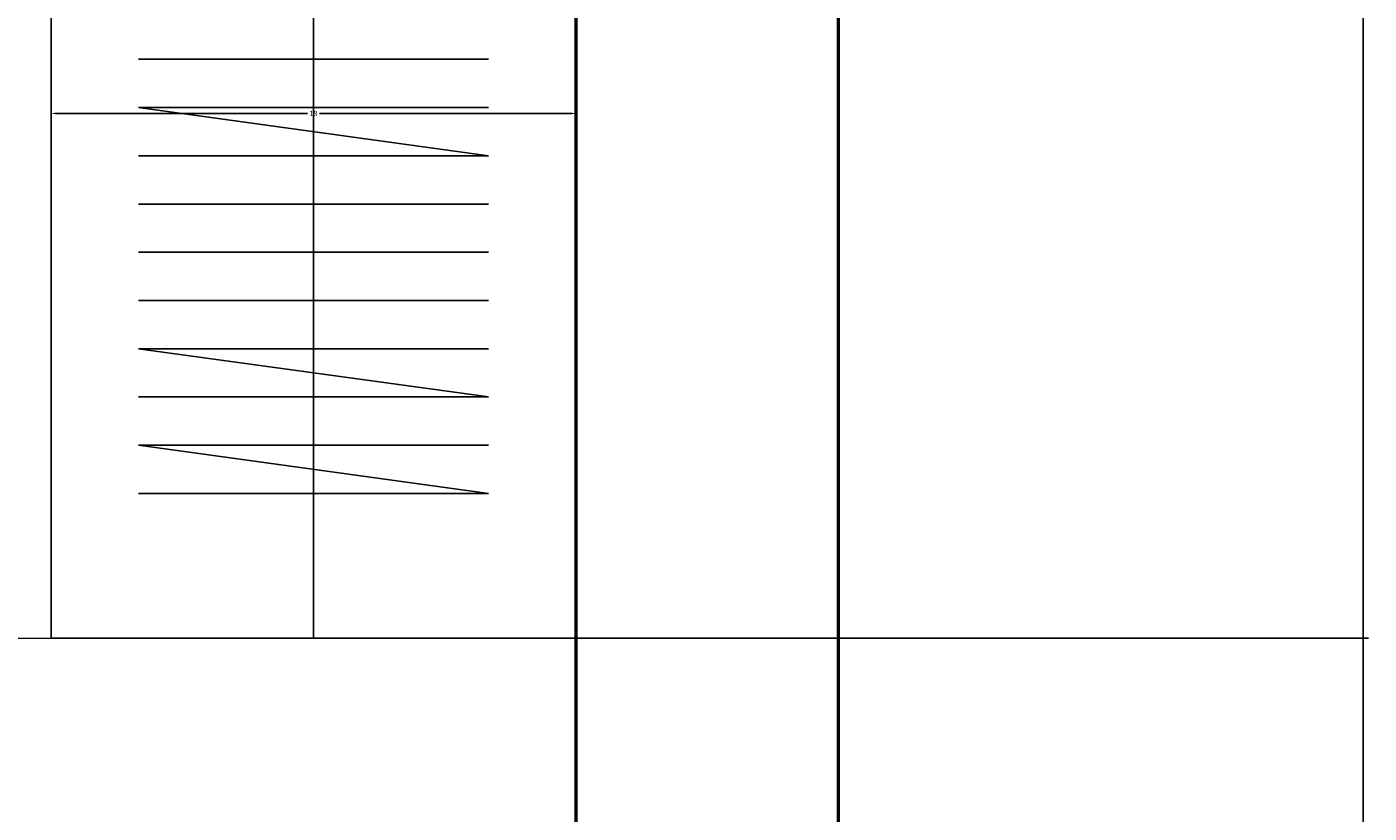
# Model space of a CAD drawing. Units: inches. Extents: x 2621 to 2849, y 2066 to 2463.
# Tile 21 of 28: x 2803 to 2849, y 2317 to 2344. Entities that reach past the tile are written whole.
import ezdxf

# ---------------------------------------------------------------- set-up
doc = ezdxf.new("R2010")
doc.units = ezdxf.units.IN
for name, color, linetype, lineweight in [('A-ANNO-DIMS', 2, 'Continuous', 18), ('A-EQPM', 8, 'Continuous', 18), ('A-FLOR-CASE', 9, 'Continuous', 25), ('A-WALL', 7, 'Continuous', 50)]:
    doc.layers.add(name, color=color, linetype=linetype, lineweight=lineweight)
doc.styles.get("Standard").update_dxf_attribs({"font": 'arial.ttf'})
doc.dimstyles.get("Standard").update_dxf_attribs({"dimtxt": 0.18, "dimasz": 0.18, "dimexe": 0.18, "dimexo": 0.0625, "dimgap": 0.09, "dimtad": 0, "dimtih": 1, "dimtoh": 1, "dimdec": 4, "dimzin": 0, "dimdsep": 46, "dimtxsty": 'Standard', "dimcen": 0.09, "dimadec": 0, "dimazin": 0, "dimtfac": 1, "dimtdec": 4, "dimtofl": 0, "dimtmove": 0, "dimatfit": 3, "dimfxl": 1, "dimtolj": 1, "dimtzin": 0, "dimarcsym": 0})

# ---------------------------------------------------------------- blocks, each defined once
blk = doc.blocks.new('Refrigerator-2 door - 36 in top')
for p, q in [((0, -26.999999), (36, -26.999999)), ((12, -26.999999), (12, -28.999999)), ((11, -27.999999), (11, -28.999999)), ((13, -28.999999), (13, -27.999999)), ((11, -28.999999), (13, -28.999999))]:
    blk.add_line(p, q)
blk.add_lwpolyline([(0, -27.999999), (0, 0), (36, 0), (36, -27.999999)], close=True)
blk = doc.blocks.new('CLOSET-HANGER')
for p, q in [((12, 1.655), (0, 1.655)), ((0, 1.655), (12, 0)), ((12, 0), (0, 0))]:
    blk.add_line(p, q)
blk = doc.blocks.new('*D36')
at = {"layer": 'A-ANNO-DIMS', "color": 0, "lineweight": -2, "transparency": 16777216}
for p, q in [((2830.933, 2444.375), (2849.054, 2444.375)), ((2848.874, 2444.195), (2848.874, 2264.557)), ((2848.874, 2084.555), (2848.874, 2264.193)), ((2830.933, 2084.375), (2849.054, 2084.375))]:
    blk.add_line(p, q, dxfattribs=at)
at = {"layer": 'A-ANNO-DIMS', "color": 0, "transparency": 16777216}
for points in [[(2848.844, 2444.195), (2848.904, 2444.195), (2848.874, 2444.375)], [(2848.844, 2084.555), (2848.904, 2084.555), (2848.874, 2084.375)]]:
    blk.add_solid(points, dxfattribs=at)
at = {"layer": 'Defpoints', "color": 0, "transparency": 16777216}
for p in [(2830.87, 2444.375), (2848.874, 2444.375), (2830.87, 2084.375)]:
    blk.add_point(p, dxfattribs=at)
at = {"layer": 'A-ANNO-DIMS', "color": 0, "transparency": 16777216, "insert": (2848.874, 2264.375), "char_height": 0.18, "attachment_point": 5}
blk.add_mtext('\\A1;360', dxfattribs=at)
blk = doc.blocks.new('*D54')
at = {"layer": 'A-ANNO-DIMS', "color": 0, "lineweight": -2, "transparency": 16777216}
for p, q in [((2821.933, 2371.375), (2849.054, 2371.375)), ((2848.874, 2371.195), (2848.874, 2347.556)), ((2848.874, 2323.555), (2848.874, 2347.193)), ((2821.933, 2323.375), (2849.054, 2323.375))]:
    blk.add_line(p, q, dxfattribs=at)
at = {"layer": 'A-ANNO-DIMS', "color": 0, "transparency": 16777216}
for points in [[(2848.844, 2371.195), (2848.904, 2371.195), (2848.874, 2371.375)], [(2848.844, 2323.555), (2848.904, 2323.555), (2848.874, 2323.375)]]:
    blk.add_solid(points, dxfattribs=at)
at = {"layer": 'Defpoints', "color": 0, "transparency": 16777216}
for p in [(2821.87, 2371.375), (2821.87, 2323.375), (2848.874, 2323.375)]:
    blk.add_point(p, dxfattribs=at)
at = {"layer": 'A-ANNO-DIMS', "color": 0, "transparency": 16777216, "insert": (2848.874, 2347.375), "char_height": 0.18, "attachment_point": 5}
blk.add_mtext('\\A1;48', dxfattribs=at)
blk = doc.blocks.new('*D55')
at = {"layer": 'A-ANNO-DIMS', "color": 0, "lineweight": -2, "transparency": 16777216}
for p, q in [((2803.87, 2323.437), (2803.87, 2341.558)), ((2804.05, 2341.378), (2812.659, 2341.378)), ((2821.69, 2341.378), (2813.081, 2341.378)), ((2821.87, 2323.437), (2821.87, 2341.558))]:
    blk.add_line(p, q, dxfattribs=at)
at = {"layer": 'A-ANNO-DIMS', "color": 0, "transparency": 16777216}
for points in [[(2804.05, 2341.408), (2804.05, 2341.348), (2803.87, 2341.378)], [(2821.69, 2341.408), (2821.69, 2341.348), (2821.87, 2341.378)]]:
    blk.add_solid(points, dxfattribs=at)
at = {"layer": 'Defpoints', "color": 0, "transparency": 16777216}
for p in [(2821.87, 2341.378), (2803.87, 2323.375), (2821.87, 2323.375)]:
    blk.add_point(p, dxfattribs=at)
at = {"layer": 'A-ANNO-DIMS', "color": 0, "transparency": 16777216, "insert": (2812.87, 2341.378), "char_height": 0.18, "attachment_point": 5}
blk.add_mtext('\\A1;18', dxfattribs=at)

msp = doc.modelspace()

# ---------------------------------------------------------------- linework, layer by layer
at = {"layer": 'A-FLOR-CASE'}
for p, q in [((2803.8701, 2371.3746), (2803.8701, 2323.3746)), ((2812.8701, 2371.3746), (2812.8701, 2323.3746)), ((2821.8701, 2323.3746), (2821.8701, 2371.3746)), ((2818.8701, 2343.2367), (2806.8701, 2343.2367)), ((2818.8701, 2338.2711), (2806.8701, 2338.2711)), ((2818.8701, 2336.616), (2806.8701, 2336.616)), ((2818.8701, 2334.9608), (2806.8701, 2334.9608)), ((2803.8701, 2323.3746), (2821.8701, 2323.3746)), ((2821.8701, 2323.3746), (2803.8701, 2323.3746))]:
    msp.add_line(p, q, dxfattribs=at)
at = {"layer": 'A-WALL'}
for q in [(2821.8701, 2319.3746), (2821.8701, 2093.3746)]:
    msp.add_line((2821.8701, 2371.3746), q, dxfattribs=at)
msp.add_lwpolyline([(2761.8701, 2084.3746), (2638.8701, 2084.3746), (2638.8701, 2444.3746), (2830.8701, 2444.3746), (2830.8701, 2084.3746), (2797.8701, 2084.3746)], dxfattribs=at)

# ---------------------------------------------------------------- block references
at = {"layer": 'A-EQPM', "rotation": 270}
msp.add_blockref('Refrigerator-2 door - 36 in top', (2821.8701, 2323.3746), dxfattribs=at)
at = {"layer": 'A-FLOR-CASE'}
for p in [(2806.87, 2339.9264), (2806.87, 2331.6506), (2806.87, 2328.3402)]:
    msp.add_blockref('CLOSET-HANGER', p, dxfattribs=at)

# ---------------------------------------------------------------- dimensions: what is measured, and where the dimension line sits
at = {"layer": 'A-ANNO-DIMS'}
for base, p1, p2, picture, middle in [((2848.8736, 2444.3746), (2830.8701, 2084.3746), (2830.8701, 2444.3746), '*D36', (2848.8736, 2264.3746)), ((2848.8736, 2323.3746), (2821.8701, 2371.3746), (2821.8701, 2323.3746), '*D54', (2848.8736, 2347.3746))]:
    dim = msp.add_linear_dim(base=base, p1=p1, p2=p2, angle=90, dimstyle='Standard', override={"dimdec": 0, "dimlfac": 1, "dimrnd": 0, "dimzin": 0, "dimdsep": 46, "dimlunit": 2}, dxfattribs=at)
    dim.commit()
    dim.dimension.update_dxf_attribs({"geometry": picture, "text_midpoint": middle})
dim = msp.add_linear_dim(base=(2821.8701, 2341.3781), p1=(2803.8701, 2323.3746), p2=(2821.8701, 2323.3746), dimstyle='Standard', override={"dimdec": 0, "dimlfac": 1, "dimrnd": 0, "dimzin": 0, "dimdsep": 46, "dimlunit": 2}, dxfattribs=at)
dim.commit()
dim.dimension.update_dxf_attribs({"geometry": '*D55', "text_midpoint": (2812.8701, 2341.3781)})

doc.saveas('drawing.dxf')
